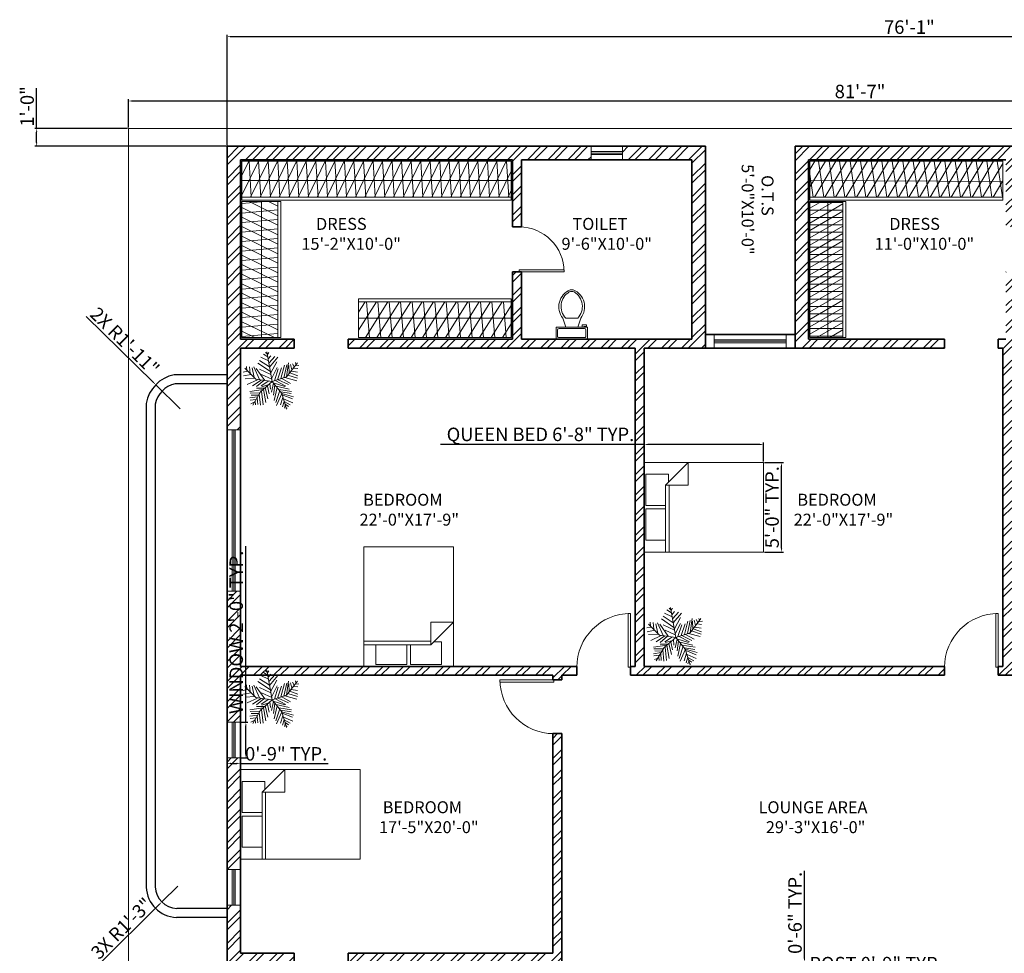
# Model space of a CAD drawing. Units: inches. Extents: x 155 to 1269, y 1260 to 2528.
# Tile 5 of 6: x 155 to 813, y 1903 to 2528. Entities that reach past the tile are written whole.
import ezdxf

# ---------------------------------------------------------------- set-up
doc = ezdxf.new("R2010")
doc.units = ezdxf.units.IN
for name, color, linetype, lineweight in [('A-ANNO-DIMS', 2, 'Continuous', 18), ('A-AREA-IDEN', 7, 'Continuous', 18), ('A-DOOR', 3, 'Continuous', 18), ('A-FLOR-CASE', 9, 'Continuous', 18), ('A-FLOR-CASE-PATT', 252, 'Continuous', 13), ('A-FLOR-EDGE', 7, 'Continuous', 25), ('A-FLOR-FIXT', 9, 'Continuous', 18), ('A-FURN', 8, 'Continuous', 18), ('A-GLAZ', 244, 'Continuous', 18), ('A-WALL', 7, 'Continuous', 35), ('A-WALL-PATT', 252, 'Continuous', 13), ('C-PROP', 8, 'Continuous', 18), ('L-PLNT', 94, 'Continuous', 13)]:
    doc.layers.add(name, color=color, linetype=linetype, lineweight=lineweight)
doc.styles.get("Standard").update_dxf_attribs({"font": 'arial.ttf'})
doc.dimstyles.new('ISO-25', dxfattribs={"dimtxt": 9, "dimasz": 2.5, "dimexe": 1.25, "dimexo": 0.625, "dimtad": 1, "dimlunit": 3, "dimtxsty": 'Standard', "dimcen": 2.5, "dimadec": 0, "dimazin": 0, "dimtfac": 1, "dimtmove": 0, "dimatfit": 3, "dimfxl": 1, "dimarcsym": 0})

# ---------------------------------------------------------------- blocks, each defined once
blk = doc.blocks.new('*U2')
for p, q in [((0, 0), (0, -6)), ((-40, 0), (-40, -6))]:
    blk.add_line(p, q)
blk.add_lwpolyline([(0, 0), (0, 40), (-1.75, 40), (-1.75, 0)], close=True)
blk.add_arc((0, 0), 40, 90, 180)
blk = doc.blocks.new('Bed - Queen')
for p, q in [((0, -80.00003), (0, 0)), ((0, 0), (59.99999, 0)), ((59.99999, 0), (59.99999, -80.00003)), ((7.99999, -1.2), (28.79998, -1.2)), ((7.99999, -14.4), (7.99999, -1.2)), ((28.79998, -1.2), (28.79998, -14.4)), ((31.19999, -1.2), (51.99999, -1.2)), ((31.19999, -14.4), (31.19999, -1.2)), ((51.99999, -1.2), (51.99999, -16.4)), ((0, -14.4), (44.8, -14.4)), ((44.8, -16.8), (0, -16.8)), ((59.99999, -29.6), (44.8, -14.4)), ((44.8, -14.4), (44.8, -29.6)), ((51.99999, -16.4), (46.79936, -16.4)), ((44.8, -29.6), (59.99999, -29.6)), ((59.99999, -80.00003), (0, -80.00003))]:
    blk.add_line(p, q)
blk = doc.blocks.new('*U8')
for p, q in [((9.5, -6), (9.5, -2)), ((-10, -8.5), (-8, -8.5)), ((-10, -9.5), (-10, -8.5)), ((-7, -9.5), (-10, -9.5)), ((-8, -8.5), (-8, -8)), ((-7, -8), (-7, -9.5)), ((-4, -8), (-6, -14)), ((4, -8), (6, -14)), ((4, -14), (-4, -14))]:
    blk.add_line(p, q)
blk.add_lwpolyline([(10.5, -8), (10.5, 0), (-10.5, 0), (-10.5, -8)], close=True)
for points in [[(-9.5, -2), (-9.5, -6)], [(8.5, -1), (-8.5, -1)], [(-8.5, -7), (8.5, -7)]]:
    blk.add_lwpolyline(points)
for centre, radius, start, end in [((-8.62, -1.88), 0.884, 81.8699, 188.1301), ((-8.62, -6.12), 0.884, 171.8699, 278.1301), ((8.62, -1.88), 0.884, 351.8699, 98.1301), ((8.62, -6.12), 0.884, 261.8699, 8.1301), ((3.52, -21.58), 12.17, 141.46911, 247.97143), ((4.2, -21.82), 11.33, 136.36773, 238.94682), ((-3.52, -21.58), 12.17, 292.02843, 38.53071), ((-4.2, -21.82), 11.33, 301.05301, 43.63209), ((0, -27.88), 4, 245.73182, 294.26817), ((0, -29), 4, 254.86053, 285.13947)]:
    blk.add_arc(centre, radius, start, end)
blk = doc.blocks.new('*U11')
for p, q in [((0, 0), (-10.5, 57)), ((-5.114, 28.097), (-24.676, 40.636)), ((-7.288, 39.707), (-21.778, 46.673)), ((-8.737, 47.138), (-17.069, 52.711)), ((-10.186, 53.64), (-13.084, 55.962)), ((-9.099, 51.782), (-6.563, 55.962)), ((-7.65, 43.423), (-2.578, 49.46)), ((-5.839, 35.992), (4.667, 48.067)), ((-5.114, 27.632), (10.463, 46.673)), ((-2.941, 16.486), (8.652, 37.85)), ((-47.498, 19.737), (-55.83, 18.344)), ((-31.5, 4.5), (-52.5, 25.5)), ((-48.585, 21.131), (-49.309, 29.026)), ((-43.513, 28.561), (-42.427, 15.558)), ((-38.442, 26.239), (-34.819, 7.663)), ((-35.544, 28.097), (-24.314, 3.947)), ((-14.533, 2.09), (-30.834, 25.31)), ((-3.665, 19.273), (-27.574, 35.527)), ((-24.314, 23.917), (-2.941, 13.7)), ((-1.129, 6.734), (9.014, 26.704)), ((3.942, 1.625), (11.187, 24.381)), ((10.101, 3.483), (17.708, 26.239)), ((16.259, 5.805), (23.142, 31.348)), ((22.055, 7.198), (27.489, 32.277)), ((27, 9), (48, 36)), ((27.127, 9.056), (31.112, 35.992)), ((31.836, 30.883), (32.561, 16.486)), ((35.096, 32.741), (37.27, 22.524)), ((36.183, 19.737), (48.137, 17.88)), ((38.719, 34.134), (41.979, 28.561)), ((40.53, 25.775), (48.862, 24.846)), ((43.791, 29.954), (51.036, 30.883)), ((44.153, 36.456), (45.239, 32.741)), ((-40.615, 13.7), (-55.105, 10.913)), ((-33.37, 6.269), (-52.207, 5.34)), ((-28.299, 3.483), (-47.86, -5.805)), ((-21.416, 3.018), (-38.079, -8.128)), ((0, 0), (-31.5, 4.5)), ((-15.982, 2.09), (-30.11, -9.521)), ((0, 0), (-22.5, -19.5)), ((-6.563, 1.161), (-21.416, -8.128)), ((-20.691, 13.7), (-1.129, 4.876)), ((0, 0), (27, 9)), ((0, 0), (18, -22.5)), ((6.478, 1.625), (26.04, -8.592)), ((11.187, 3.483), (30.749, -5.805)), ((18.07, 5.805), (35.096, -3.483)), ((24.229, 7.663), (46.688, 1.625)), ((29.662, 12.307), (48.137, 6.269)), ((33.285, 16.486), (48.862, 10.913)), ((-17.431, -15.094), (-42.789, -18.809)), ((-15.257, -12.772), (-30.11, -12.772)), ((-20.691, -18.345), (-17.793, -44.352)), ((-6.563, -5.805), (-19.967, -9.985)), ((-17.069, -15.094), (-12.721, -40.172)), ((-13.446, -11.378), (-8.737, -32.741)), ((-9.461, -8.592), (-6.201, -23.453)), ((-4.752, -3.483), (-3.665, -14.629)), ((2.493, -3.019), (-1.491, -20.202)), ((1.769, -2.555), (24.229, -9.521)), ((5.029, -6.27), (2.131, -25.775)), ((9.014, -11.378), (3.58, -35.992)), ((14.085, -16.951), (6.478, -40.172)), ((7.565, -9.056), (32.198, -14.629)), ((12.274, -15.094), (36.907, -18.809)), ((-28.299, -29.026), (-42.789, -31.348)), ((-24.314, -21.596), (-42.427, -22.06)), ((-30.834, -34.135), (-42.427, -35.528)), ((-26.849, -26.24), (-40.253, -25.775)), ((-22.5, -19.5), (-37.5, -45)), ((-32.646, -36.921), (-31.921, -44.352)), ((-29.023, -30.884), (-27.936, -43.887)), ((-25.038, -23.918), (-22.865, -45.281)), ((18.07, -22.524), (8.289, -45.745)), ((20.244, -30.419), (15.897, -44.816)), ((16.259, -19.738), (36.183, -22.989)), ((18, -22.5), (27, -52.5)), ((18.433, -22.524), (40.53, -29.026)), ((19.157, -25.311), (38.719, -33.206)), ((21.331, -32.741), (39.081, -40.636)), ((-34.457, -39.708), (-40.978, -42.494)), ((22.78, -37.85), (19.519, -48.532)), ((22.78, -38.314), (34.372, -44.816)), ((24.591, -45.745), (23.142, -50.854)), ((24.591, -43.423), (30.749, -47.603)), ((26.764, -49.925), (28.213, -50.854))]:
    blk.add_line(p, q)
blk = doc.blocks.new('*D12')
at = {"layer": 'A-ANNO-DIMS', "color": 0, "lineweight": -2, "transparency": 16777216}
for p, q in [((227.4, 2455.81), (227.4, 2474.72)), ((1203.9, 2473.47), (229.9, 2473.47)), ((1206.4, 2455.81), (1206.4, 2474.72))]:
    blk.add_line(p, q, dxfattribs=at)
at = {"layer": 'A-ANNO-DIMS', "color": 0, "transparency": 16777216}
for points in [[(229.9, 2473.89), (229.9, 2473.06), (227.4, 2473.47)], [(1203.9, 2473.89), (1203.9, 2473.06), (1206.4, 2473.47)]]:
    blk.add_solid(points, dxfattribs=at)
at = {"layer": 'Defpoints', "color": 0, "transparency": 16777216}
for p in [(227.4, 2473.47), (227.4, 2455.18), (1206.4, 2455.18)]:
    blk.add_point(p, dxfattribs=at)
at = {"layer": 'A-ANNO-DIMS', "color": 0, "transparency": 16777216, "insert": (716.9, 2478.69), "char_height": 9, "attachment_point": 5}
blk.add_mtext('81\'-7"', dxfattribs=at)
blk = doc.blocks.new('WIN-21IN')
for p, q in [((21, 5.5), (0, 5.5)), ((21, 4.5), (0, 4.5)), ((21, 3.5), (0, 3.5))]:
    blk.add_line(p, q)
blk.add_lwpolyline([(0, 9), (21, 9), (21, 0), (0, 0)], close=True)
blk = doc.blocks.new('WIN-108IN')
for p, q in [((3.5, 108), (3.5, 0)), ((4.5, 108), (4.5, 0)), ((5.5, 108), (5.5, 0))]:
    blk.add_line(p, q)
blk.add_lwpolyline([(9, 108), (9, 0), (0, 0), (0, 108)], close=True)
blk = doc.blocks.new('WIN-24IN')
for p, q in [((3.5, 24), (3.5, 0)), ((4.5, 24), (4.5, 0)), ((5.5, 24), (5.5, 0))]:
    blk.add_line(p, q)
blk.add_lwpolyline([(0, 24), (9, 24), (9, 0), (0, 0)], close=True)
blk = doc.blocks.new('WIN-48IN')
for p, q in [((0, 5.5), (48, 5.5)), ((0, 4.5), (48, 4.5)), ((0, 3.5), (48, 3.5))]:
    blk.add_line(p, q)
blk.add_lwpolyline([(0, 9), (48, 9), (48, 0), (0, 0)], close=True)
blk = doc.blocks.new('*D22')
at = {"layer": 'A-ANNO-DIMS', "color": 0, "lineweight": -2, "transparency": 16777216}
for p, q in [((572.4, 2243.68), (436.26, 2243.68)), ((572.4, 2232.31), (572.4, 2244.93)), ((649.9, 2243.68), (574.9, 2243.68)), ((652.4, 2232.31), (652.4, 2244.93))]:
    blk.add_line(p, q, dxfattribs=at)
at = {"layer": 'A-ANNO-DIMS', "color": 0, "transparency": 16777216}
for points in [[(574.9, 2244.1), (574.9, 2243.26), (572.4, 2243.68)], [(649.9, 2244.1), (649.9, 2243.26), (652.4, 2243.68)]]:
    blk.add_solid(points, dxfattribs=at)
at = {"layer": 'Defpoints', "color": 0, "transparency": 16777216}
for p in [(572.4, 2243.68), (572.4, 2231.68), (652.4, 2231.68)]:
    blk.add_point(p, dxfattribs=at)
at = {"layer": 'A-ANNO-DIMS', "color": 0, "transparency": 16777216, "insert": (503.08, 2249.24), "char_height": 9, "attachment_point": 5}
blk.add_mtext('QUEEN BED 6\'-8" TYP.', dxfattribs=at)
blk = doc.blocks.new('*D23')
at = {"layer": 'A-ANNO-DIMS', "color": 0, "lineweight": -2, "transparency": 16777216}
for p, q in [((653.02, 2231.68), (665.65, 2231.68)), ((664.4, 2174.18), (664.4, 2229.18)), ((653.02, 2171.68), (665.65, 2171.68))]:
    blk.add_line(p, q, dxfattribs=at)
at = {"layer": 'A-ANNO-DIMS', "color": 0, "transparency": 16777216}
for points in [[(663.98, 2229.18), (664.81, 2229.18), (664.4, 2231.68)], [(663.98, 2174.18), (664.81, 2174.18), (664.4, 2171.68)]]:
    blk.add_solid(points, dxfattribs=at)
at = {"layer": 'Defpoints', "color": 0, "transparency": 16777216}
for p in [(652.4, 2231.68), (664.4, 2231.68), (652.4, 2171.68)]:
    blk.add_point(p, dxfattribs=at)
at = {"layer": 'A-ANNO-DIMS', "color": 0, "transparency": 16777216, "insert": (659.18, 2201.68), "char_height": 9, "attachment_point": 5, "rotation": 90}
blk.add_mtext('5\'-0" TYP.', dxfattribs=at)
blk = doc.blocks.new('*D26')
at = {"layer": 'A-ANNO-DIMS', "color": 0, "lineweight": -2, "transparency": 16777216}
for p, q in [((669.4, 1890.56), (669.4, 1888.58)), ((678.4, 1890.56), (678.4, 1888.58)), ((671.9, 1889.83), (675.9, 1889.83)), ((678.4, 1889.83), (774.28, 1889.83))]:
    blk.add_line(p, q, dxfattribs=at)
at = {"layer": 'A-ANNO-DIMS', "color": 0, "transparency": 16777216}
for points in [[(671.9, 1890.25), (671.9, 1889.41), (669.4, 1889.83)], [(675.9, 1890.25), (675.9, 1889.41), (678.4, 1889.83)]]:
    blk.add_solid(points, dxfattribs=at)
at = {"layer": 'Defpoints', "color": 0, "transparency": 16777216}
for p in [(669.4, 1891.18), (678.4, 1891.18), (678.4, 1889.83)]:
    blk.add_point(p, dxfattribs=at)
at = {"layer": 'A-ANNO-DIMS', "color": 0, "transparency": 16777216, "insert": (727.59, 1895.11), "char_height": 9, "attachment_point": 5}
blk.add_mtext('POST 0\'-9" TYP.', dxfattribs=at)
blk = doc.blocks.new('*D27')
at = {"layer": 'A-ANNO-DIMS', "color": 0, "lineweight": -2, "transparency": 16777216}
for p, q in [((679.75, 1899.68), (679.75, 1958.29)), ((679.02, 1897.18), (681, 1897.18)), ((679.75, 1891.18), (679.75, 1897.18)), ((679.02, 1891.18), (681, 1891.18)), ((679.75, 1888.68), (679.75, 1886.18))]:
    blk.add_line(p, q, dxfattribs=at)
at = {"layer": 'A-ANNO-DIMS', "color": 0, "transparency": 16777216}
for points in [[(679.33, 1899.68), (680.16, 1899.68), (679.75, 1897.18)], [(679.33, 1888.68), (680.16, 1888.68), (679.75, 1891.18)]]:
    blk.add_solid(points, dxfattribs=at)
at = {"layer": 'Defpoints', "color": 0, "transparency": 16777216}
for p in [(678.4, 1897.18), (679.75, 1897.18), (678.4, 1891.18)]:
    blk.add_point(p, dxfattribs=at)
at = {"layer": 'A-ANNO-DIMS', "color": 0, "transparency": 16777216, "insert": (674.53, 1930.24), "char_height": 9, "attachment_point": 5, "rotation": 90}
blk.add_mtext('0\'-6" TYP.', dxfattribs=at)
blk = doc.blocks.new('*D32')
at = {"layer": 'A-ANNO-DIMS', "color": 0, "lineweight": -2, "transparency": 16777216}
for p, q in [((306, 2057.89), (306, 2175.53)), ((303.02, 2057.89), (307.25, 2057.89)), ((306, 2036.39), (306, 2055.39)), ((303.02, 2033.89), (307.25, 2033.89))]:
    blk.add_line(p, q, dxfattribs=at)
at = {"layer": 'A-ANNO-DIMS', "color": 0, "transparency": 16777216}
for points in [[(305.58, 2055.39), (306.41, 2055.39), (306, 2057.89)], [(305.58, 2036.39), (306.41, 2036.39), (306, 2033.89)]]:
    blk.add_solid(points, dxfattribs=at)
at = {"layer": 'Defpoints', "color": 0, "transparency": 16777216}
for p in [(302.4, 2057.89), (306, 2057.89), (302.4, 2033.89)]:
    blk.add_point(p, dxfattribs=at)
at = {"layer": 'A-ANNO-DIMS', "color": 0, "transparency": 16777216, "insert": (300.72, 2117.96), "char_height": 9, "attachment_point": 5, "rotation": 90}
blk.add_mtext('WINDOW 2\'-0" TYP.', dxfattribs=at)
blk = doc.blocks.new('*D33')
at = {"layer": 'A-ANNO-DIMS', "color": 0, "lineweight": -2, "transparency": 16777216}
for p, q in [((293.4, 2033.27), (293.4, 2029.04)), ((295.9, 2030.29), (299.9, 2030.29)), ((302.4, 2033.27), (302.4, 2029.04)), ((302.4, 2030.29), (361.01, 2030.29))]:
    blk.add_line(p, q, dxfattribs=at)
at = {"layer": 'A-ANNO-DIMS', "color": 0, "transparency": 16777216}
for points in [[(295.9, 2030.71), (295.9, 2029.87), (293.4, 2030.29)], [(299.9, 2030.71), (299.9, 2029.87), (302.4, 2030.29)]]:
    blk.add_solid(points, dxfattribs=at)
at = {"layer": 'Defpoints', "color": 0, "transparency": 16777216}
for p in [(293.4, 2033.89), (302.4, 2033.89), (302.4, 2030.29)]:
    blk.add_point(p, dxfattribs=at)
at = {"layer": 'A-ANNO-DIMS', "color": 0, "transparency": 16777216, "insert": (332.95, 2035.51), "char_height": 9, "attachment_point": 5}
blk.add_mtext('0\'-9" TYP.', dxfattribs=at)
blk = doc.blocks.new('*D42')
at = {"layer": 'A-ANNO-DIMS', "color": 0, "lineweight": -2, "transparency": 16777216}
for p, q in [((293.4, 2443.81), (293.4, 2517.78)), ((295.9, 2516.53), (1203.9, 2516.53)), ((1206.4, 2443.81), (1206.4, 2517.78))]:
    blk.add_line(p, q, dxfattribs=at)
at = {"layer": 'A-ANNO-DIMS', "color": 0, "transparency": 16777216}
for points in [[(295.9, 2516.95), (295.9, 2516.11), (293.4, 2516.53)], [(1203.9, 2516.95), (1203.9, 2516.11), (1206.4, 2516.53)]]:
    blk.add_solid(points, dxfattribs=at)
at = {"layer": 'Defpoints', "color": 0, "transparency": 16777216}
for p in [(1206.4, 2516.53), (293.4, 2443.18), (1206.4, 2443.18)]:
    blk.add_point(p, dxfattribs=at)
at = {"layer": 'A-ANNO-DIMS', "color": 0, "transparency": 16777216, "insert": (749.9, 2521.75), "char_height": 9, "attachment_point": 5}
blk.add_mtext('76\'-1"', dxfattribs=at)
blk = doc.blocks.new('*D43')
at = {"layer": 'A-ANNO-DIMS', "color": 0, "lineweight": -2, "transparency": 16777216}
for p, q in [((166.05, 2455.18), (166.05, 2482.01)), ((226.77, 2455.18), (164.8, 2455.18)), ((166.05, 2445.68), (166.05, 2452.68)), ((292.77, 2443.18), (164.8, 2443.18))]:
    blk.add_line(p, q, dxfattribs=at)
at = {"layer": 'A-ANNO-DIMS', "color": 0, "transparency": 16777216}
for points in [[(165.63, 2452.68), (166.46, 2452.68), (166.05, 2455.18)], [(165.63, 2445.68), (166.46, 2445.68), (166.05, 2443.18)]]:
    blk.add_solid(points, dxfattribs=at)
at = {"layer": 'Defpoints', "color": 0, "transparency": 16777216}
for p in [(166.05, 2455.18), (227.4, 2455.18), (293.4, 2443.18)]:
    blk.add_point(p, dxfattribs=at)
at = {"layer": 'A-ANNO-DIMS', "color": 0, "transparency": 16777216, "insert": (160.83, 2469.84), "char_height": 9, "attachment_point": 5, "rotation": 90}
blk.add_mtext('1\'-0"', dxfattribs=at)
blk = doc.blocks.new('*D50')
at = {"layer": 'A-ANNO-DIMS', "color": 0, "lineweight": -2, "transparency": 16777216}
for p, q in [((199.11, 2329.37), (243.91, 2285.4)), ((262.1, 2267.55), (245.69, 2283.65))]:
    blk.add_line(p, q, dxfattribs=at)
at = {"layer": 'A-ANNO-DIMS', "color": 0, "transparency": 16777216}
blk.add_solid([(244.2, 2285.7), (243.62, 2285.1), (245.69, 2283.65)], dxfattribs=at)
at = {"layer": 'Defpoints', "color": 0, "transparency": 16777216}
for p in [(245.69, 2283.65), (262.1, 2267.55)]:
    blk.add_point(p, dxfattribs=at)
at = {"layer": 'A-ANNO-DIMS', "color": 0, "transparency": 16777216, "insert": (224.22, 2311.93), "char_height": 9, "attachment_point": 5, "rotation": 315.54002}
blk.add_mtext('2X R1\'-11"', dxfattribs=at)
blk = doc.blocks.new('*D56')
at = {"layer": 'A-ANNO-DIMS', "color": 0, "lineweight": -2, "transparency": 16777216}
for p, q in [((260.38, 1948.16), (249.76, 1937.58)), ((208.58, 1896.56), (247.98, 1935.81))]:
    blk.add_line(p, q, dxfattribs=at)
at = {"layer": 'A-ANNO-DIMS', "color": 0, "transparency": 16777216}
blk.add_solid([(247.69, 1936.11), (248.28, 1935.52), (249.76, 1937.58)], dxfattribs=at)
at = {"layer": 'Defpoints', "color": 0, "transparency": 16777216}
for p in [(260.38, 1948.16), (249.76, 1937.58)]:
    blk.add_point(p, dxfattribs=at)
at = {"layer": 'A-ANNO-DIMS', "color": 0, "transparency": 16777216, "insert": (223.71, 1919), "char_height": 9, "attachment_point": 5, "rotation": 44.89223}
blk.add_mtext('3X R1\'-3"', dxfattribs=at)

msp = doc.modelspace()

# ---------------------------------------------------------------- hatches: boundary and pattern name
at = {"layer": 'A-FLOR-CASE-PATT'}
h = msp.add_hatch(dxfattribs=at)
h.set_pattern_fill('ANSI31', color=256, scale=1.80661, angle=19.0965, style=0)
h.paths.add_polyline_path([(303.397, 2409.181), (483.397, 2409.181), (483.397, 2433.181), (303.397, 2433.181)])
h = msp.add_hatch(dxfattribs=at)
h.set_pattern_fill('ANSI31', color=256, scale=2.00453, angle=48.55, style=0)
h.paths.add_polyline_path([(303.397, 2409.181), (483.397, 2409.181), (483.397, 2433.181), (303.397, 2433.181)])
h = msp.add_hatch(dxfattribs=at)
h.set_pattern_fill('ANSI31', color=256, scale=1.89921, angle=14.0303, style=0)
h.paths.add_polyline_path([(683.397, 2409.181), (812.397, 2409.181), (812.397, 2433.181), (683.397, 2433.181)])
h = msp.add_hatch(dxfattribs=at)
h.set_pattern_fill('ANSI31', color=256, scale=2.1922, angle=53.2238, style=0)
h.paths.add_polyline_path([(683.397, 2409.181), (812.397, 2409.181), (812.397, 2433.181), (683.397, 2433.181)])
h = msp.add_hatch(dxfattribs=at)
h.set_pattern_fill('ANSI31', color=256, scale=1.799134, angle=108.8969, style=0)
h.paths.add_polyline_path([(303.397, 2315.181), (327.397, 2315.181), (327.397, 2406.181), (303.397, 2406.181)])
h = msp.add_hatch(dxfattribs=at)
h.set_pattern_fill('ANSI31', color=256, scale=1.99625, angle=-40.1304, style=0)
h.paths.add_polyline_path([(303.397, 2315.181), (327.397, 2315.181), (327.397, 2406.181), (303.397, 2406.181)])
h = msp.add_hatch(dxfattribs=at)
h.set_pattern_fill('ANSI31', color=256, scale=1.349876, angle=-14.7838, style=0)
h.paths.add_polyline_path([(683.397, 2315.181), (705.397, 2315.181), (705.397, 2406.181), (683.397, 2406.181)])
h = msp.add_hatch(dxfattribs=at)
h.set_pattern_fill('ANSI31', color=256, scale=1.562117, angle=-45, style=0)
h.paths.add_polyline_path([(683.397, 2315.181), (705.397, 2315.181), (705.397, 2406.181), (683.397, 2406.181)])
h = msp.add_hatch(dxfattribs=at)
h.set_pattern_fill('ANSI31', color=256, scale=2.03916, angle=12.988, style=0)
h.paths.add_polyline_path([(381.458, 2315.181), (483.397, 2315.181), (483.397, 2339.181), (381.458, 2339.181)])
h = msp.add_hatch(dxfattribs=at)
h.set_pattern_fill('ANSI31', color=256, scale=2.39665, angle=49.7328, style=0)
h.paths.add_polyline_path([(381.458, 2315.181), (483.397, 2315.181), (483.397, 2339.181), (381.458, 2339.181)])
at = {"layer": 'A-WALL-PATT'}
h = msp.add_hatch(dxfattribs=at)
h.set_pattern_fill('ANSI32', color=256)
h.paths.add_polyline_path([(614.897, 1534.181), (593.397, 1534.181), (593.397, 1555.181), (589.397, 1555.181), (589.397, 1534.181), (517.397, 1534.181), (517.397, 1555.181), (511.397, 1555.181), (511.397, 1495.181), (488.631, 1495.181), (488.631, 1486.181), (517.397, 1486.181), (517.397, 1525.181), (614.897, 1525.181)])
h.paths.add_polyline_path([(440.631, 1495.181), (344.954, 1495.181), (344.954, 1486.181), (440.631, 1486.181)])
h.paths.add_polyline_path([(323.954, 1495.181), (302.397, 1495.181), (302.397, 1625.863), (332.397, 1625.863), (332.397, 1631.863), (302.397, 1631.863), (302.397, 1634.984), (293.397, 1634.984), (293.397, 1486.181), (323.954, 1486.181)])
h.paths.add_polyline_path([(302.397, 1753.181), (386.397, 1753.181), (386.397, 1726.181), (392.397, 1726.181), (392.397, 1753.181), (511.397, 1753.181), (511.397, 1693.181), (392.397, 1693.181), (392.397, 1696.181), (386.397, 1696.181), (386.397, 1693.181), (368.397, 1693.181), (368.397, 1687.181), (511.397, 1687.181), (511.397, 1663.181), (517.397, 1663.181), (517.397, 1891.181), (539.397, 1891.181), (539.397, 1897.181), (517.397, 1897.181), (517.397, 2050.181), (511.397, 2050.181), (511.397, 1903.181), (374.397, 1903.181), (374.397, 1897.181), (410.397, 1897.181), (410.397, 1843.181), (416.397, 1843.181), (416.397, 1897.181), (511.397, 1897.181), (511.397, 1759.181), (416.397, 1759.181), (416.397, 1813.181), (410.397, 1813.181), (410.397, 1759.181), (302.397, 1759.181), (302.397, 1897.181), (338.397, 1897.181), (338.397, 1903.181), (302.397, 1903.181), (302.397, 1935.29), (293.397, 1935.29), (293.397, 1682.984), (302.397, 1682.984), (302.397, 1687.181), (338.397, 1687.181), (338.397, 1693.181), (302.397, 1693.181)])
h.paths.add_polyline_path([(645.397, 1897.181), (623.397, 1897.181), (623.397, 1891.181), (645.397, 1891.181)])
h.paths.add_polyline_path([(678.397, 1897.181), (669.397, 1897.181), (669.397, 1891.181), (678.397, 1891.181)])
h.paths.add_polyline_path([(696.397, 1897.181), (687.397, 1897.181), (687.397, 1891.181), (696.397, 1891.181)])
h.paths.add_polyline_path([(714.397, 1897.181), (705.397, 1897.181), (705.397, 1891.181), (714.397, 1891.181)])
h.paths.add_polyline_path([(732.397, 1897.181), (723.397, 1897.181), (723.397, 1891.181), (732.397, 1891.181)])
h.paths.add_polyline_path([(302.397, 2033.891), (293.397, 2033.891), (293.397, 1959.29), (302.397, 1959.29)], flags=17)
h.paths.add_polyline_path([(302.397, 2089.181), (511.397, 2089.181), (511.397, 2086.181), (517.397, 2086.181), (517.397, 2089.181), (527.397, 2089.181), (527.397, 2095.181), (302.397, 2095.181), (302.397, 2145.471), (293.397, 2145.471), (293.397, 2057.891), (302.397, 2057.891)])
h.paths.add_polyline_path([(773.397, 2095.181), (572.397, 2095.181), (572.397, 2308.181), (613.397, 2308.181), (613.397, 2443.181), (557.897, 2443.181), (557.897, 2434.181), (604.397, 2434.181), (604.397, 2314.181), (490.397, 2314.181), (490.397, 2359.181), (484.397, 2359.181), (484.397, 2314.181), (374.397, 2314.181), (374.397, 2308.181), (566.397, 2308.181), (566.397, 2095.181), (563.397, 2095.181), (563.397, 2089.181), (773.397, 2089.181)])
h.paths.add_polyline_path([(1070.397, 2147.681), (1061.397, 2147.681), (1061.397, 2095.181), (857.397, 2095.181), (857.397, 2089.181), (868.397, 2089.181), (868.397, 2086.181), (874.397, 2086.181), (874.397, 2089.181), (1061.397, 2089.181), (1061.397, 2050.181), (1070.397, 2050.181)])
h.paths.add_polyline_path([(821.397, 2095.181), (818.397, 2095.181), (818.397, 2308.181), (1022.397, 2308.181), (1022.397, 2314.181), (940.397, 2314.181), (940.397, 2434.181), (1077.397, 2434.181), (1077.397, 2389.181), (1083.397, 2389.181), (1083.397, 2434.181), (1129.897, 2434.181), (1129.897, 2443.181), (887.897, 2443.181), (887.897, 2434.181), (934.397, 2434.181), (934.397, 2314.181), (820.397, 2314.181), (820.397, 2359.181), (814.397, 2359.181), (814.397, 2314.181), (809.397, 2314.181), (809.397, 2308.181), (812.397, 2308.181), (812.397, 2095.181), (809.397, 2095.181), (809.397, 2089.181), (821.397, 2089.181)])
h.paths.add_polyline_path([(874.397, 2050.181), (868.397, 2050.181), (868.397, 1741.181), (877.397, 1741.181), (877.397, 1747.181), (892.397, 1747.181), (892.397, 1753.181), (874.397, 1753.181), (874.397, 1819.181), (940.397, 1819.181), (940.397, 1753.181), (922.397, 1753.181), (922.397, 1747.181), (946.397, 1747.181), (946.397, 1819.181), (1151.397, 1819.181), (1151.397, 1683.181), (931.397, 1683.181), (931.397, 1677.181), (1064.397, 1677.181), (1064.397, 1495.181), (877.397, 1495.181), (877.397, 1638.181), (868.397, 1638.181), (868.397, 1534.181), (796.397, 1534.181), (796.397, 1555.181), (792.397, 1555.181), (792.397, 1534.181), (770.897, 1534.181), (770.897, 1525.181), (868.397, 1525.181), (868.397, 1486.181), (1073.397, 1486.181), (1073.397, 1677.181), (1160.397, 1677.181), (1160.397, 1825.181), (1070.397, 1825.181), (1070.397, 1942.181), (1061.397, 1942.181), (1061.397, 1903.181), (913.397, 1903.181), (913.397, 1897.181), (1061.397, 1897.181), (1061.397, 1825.181), (957.406, 1825.181), (957.406, 1861.181), (951.406, 1861.181), (951.406, 1825.181), (874.397, 1825.181), (874.397, 1897.181), (877.397, 1897.181), (877.397, 1903.181), (874.397, 1903.181)])
h.paths.add_polyline_path([(1070.397, 2305.181), (1206.397, 2305.181), (1206.397, 2443.181), (1150.897, 2443.181), (1150.897, 2434.181), (1197.397, 2434.181), (1197.397, 2314.181), (1083.397, 2314.181), (1083.397, 2359.181), (1077.397, 2359.181), (1077.397, 2314.181), (1058.397, 2314.181), (1058.397, 2308.181), (1061.397, 2308.181), (1061.397, 2255.681), (1070.397, 2255.681)])
h.paths.add_polyline_path([(866.897, 2443.181), (673.397, 2443.181), (673.397, 2308.181), (773.397, 2308.181), (773.397, 2314.181), (682.397, 2314.181), (682.397, 2434.181), (814.397, 2434.181), (814.397, 2389.181), (818.897, 2389.181), (820.397, 2389.181), (820.397, 2434.181), (866.897, 2434.181)])
h.paths.add_polyline_path([(536.897, 2443.181), (293.397, 2443.181), (293.397, 2253.471), (302.397, 2253.471), (302.397, 2308.181), (338.397, 2308.181), (338.397, 2314.181), (302.397, 2314.181), (302.397, 2434.181), (484.397, 2434.181), (484.397, 2389.181), (490.397, 2389.181), (490.397, 2434.181), (536.897, 2434.181)])

# ---------------------------------------------------------------- linework, layer by layer
at = {"layer": 'A-FLOR-CASE'}
for p, q in [((303.397, 2433.181), (483.397, 2433.181)), ((303.397, 2433.181), (303.397, 2407.181)), ((483.397, 2433.181), (483.397, 2407.181)), ((683.397, 2433.181), (812.397, 2433.181)), ((683.397, 2433.181), (683.397, 2407.181)), ((812.397, 2433.181), (812.397, 2407.181)), ((303.397, 2420.181), (483.397, 2420.181)), ((683.397, 2420.181), (812.397, 2419.681)), ((303.397, 2409.181), (483.397, 2409.181)), ((303.397, 2407.181), (483.397, 2407.181)), ((303.397, 2406.181), (329.397, 2406.181)), ((303.397, 2406.181), (303.397, 2315.181)), ((316.397, 2406.181), (316.397, 2315.181)), ((327.397, 2406.181), (327.397, 2315.181)), ((329.397, 2406.181), (329.397, 2315.181)), ((683.397, 2409.181), (812.397, 2409.181)), ((683.397, 2407.181), (812.397, 2407.181)), ((683.397, 2406.181), (707.397, 2406.181)), ((683.397, 2406.181), (683.397, 2315.181)), ((695.397, 2406.181), (695.397, 2315.181)), ((705.397, 2406.181), (705.397, 2315.181)), ((707.397, 2406.181), (707.397, 2315.181)), ((381.458, 2341.181), (483.397, 2341.181)), ((381.458, 2315.181), (381.458, 2341.181)), ((381.458, 2339.181), (483.397, 2339.181)), ((483.397, 2341.181), (483.397, 2315.181)), ((381.458, 2328.181), (483.397, 2328.181)), ((303.397, 2315.181), (329.397, 2315.181)), ((381.458, 2315.181), (483.397, 2315.181)), ((683.397, 2315.181), (707.397, 2315.181))]:
    msp.add_line(p, q, dxfattribs=at)
at = {"layer": 'A-FLOR-EDGE'}
for p, q in [((293.397, 2290.181), (258.058, 2290.181)), ((293.397, 2284.181), (258.631, 2284.181)), ((239.397, 2271.165), (239.397, 1947.446)), ((245.397, 2270.654), (245.397, 1947.556)), ((293.397, 1933.181), (259.719, 1933.181)), ((293.397, 1927.181), (259.599, 1927.181))]:
    msp.add_line(p, q, dxfattribs=at)
for centre, radius, start, end in [((262.105, 2267.546), 22.994, 100.135609, 170.943187), ((262.105, 2267.546), 16.994, 101.795322, 169.461113), ((260.376, 1948.157), 20.991, 181.941445, 267.878551), ((260.376, 1948.157), 14.991, 182.2974, 267.489584)]:
    msp.add_arc(centre, radius, start, end, dxfattribs=at)
at = {"layer": 'A-WALL'}
for p, q in [((293.397, 2443.181), (293.397, 1486.181)), ((293.397, 2443.181), (613.397, 2443.181)), ((613.397, 2443.181), (613.397, 2308.181)), ((673.397, 2443.181), (673.397, 2308.181)), ((673.397, 2443.181), (1206.397, 2443.181)), ((302.397, 2434.181), (302.397, 2314.181)), ((302.397, 2434.181), (484.397, 2434.181)), ((484.397, 2434.181), (484.397, 2389.181)), ((490.397, 2434.181), (490.397, 2389.181)), ((490.397, 2434.181), (604.397, 2434.181)), ((604.397, 2434.181), (604.397, 2314.181)), ((682.397, 2434.181), (682.397, 2314.181)), ((682.397, 2434.181), (814.397, 2434.181)), ((484.397, 2389.181), (490.397, 2389.181)), ((484.397, 2359.181), (490.397, 2359.181)), ((484.397, 2359.181), (484.397, 2314.181)), ((490.397, 2359.181), (490.397, 2314.181)), ((302.397, 2314.181), (338.397, 2314.181)), ((338.397, 2314.181), (338.397, 2308.181)), ((374.397, 2314.181), (374.397, 2308.181)), ((374.397, 2314.181), (484.397, 2314.181)), ((490.397, 2314.181), (604.397, 2314.181)), ((613.397, 2317.181), (673.397, 2317.181)), ((682.397, 2314.181), (773.397, 2314.181)), ((773.397, 2308.181), (773.397, 2314.181)), ((809.397, 2308.181), (809.397, 2314.181)), ((809.397, 2314.181), (814.397, 2314.181)), ((302.397, 2308.181), (338.397, 2308.181)), ((302.397, 2308.181), (302.397, 2095.181)), ((374.397, 2308.181), (566.397, 2308.181)), ((566.397, 2308.181), (566.397, 2095.181)), ((572.397, 2308.181), (572.397, 2095.181)), ((572.397, 2308.181), (773.397, 2308.181)), ((809.397, 2308.181), (812.397, 2308.181)), ((812.397, 2308.181), (812.397, 2095.181)), ((302.397, 2095.181), (527.397, 2095.181)), ((527.397, 2095.181), (527.397, 2089.181)), ((563.397, 2095.181), (563.397, 2089.181)), ((563.397, 2095.181), (566.397, 2095.181)), ((572.397, 2095.181), (773.397, 2095.181)), ((773.397, 2095.181), (773.397, 2089.181)), ((809.397, 2095.181), (809.397, 2089.181)), ((809.397, 2095.181), (812.397, 2095.181)), ((302.397, 2089.181), (511.397, 2089.181)), ((302.397, 2089.181), (302.397, 1903.181)), ((511.397, 2089.181), (511.397, 2086.181)), ((517.397, 2089.181), (517.397, 2086.181)), ((517.397, 2089.181), (527.397, 2089.181)), ((563.397, 2089.181), (773.397, 2089.181)), ((809.397, 2089.181), (821.397, 2089.181)), ((517.397, 2086.181), (511.397, 2086.181)), ((517.397, 2050.181), (511.397, 2050.181)), ((511.397, 2050.181), (511.397, 1903.181)), ((517.397, 2050.181), (517.397, 1897.181)), ((302.397, 1903.181), (338.397, 1903.181)), ((338.397, 1897.181), (338.397, 1903.181)), ((374.397, 1897.181), (374.397, 1903.181)), ((374.397, 1903.181), (511.397, 1903.181))]:
    msp.add_line(p, q, dxfattribs=at)
at = {"layer": 'C-PROP'}
for q in [(227.397, 1339.181), (1206.397, 2455.181)]:
    msp.add_line((227.397, 2455.181), q, dxfattribs=at)

# ---------------------------------------------------------------- block references
at = {"layer": 'A-DOOR'}
for p, xscale, yscale, zscale, rotation in [((488.897, 2359.181), 0.7500000000000114, 0.7500000000000114, 0.7500000000000114, 270), ((511.997, 2086.181), 0.9, 0.9, 0.9, 90)]:
    msp.add_blockref('*U2', p, dxfattribs=dict(at, xscale=xscale, yscale=yscale, zscale=zscale, rotation=rotation))
at = {"layer": 'A-DOOR', "xscale": 0.9, "yscale": 0.9, "zscale": 0.9}
for p in [(563.397, 2094.581), (809.397, 2094.581)]:
    msp.add_blockref('*U2', p, dxfattribs=at)
at = {"layer": 'A-FLOR-FIXT', "rotation": 180}
msp.add_blockref('*U8', (523.996, 2314.181), dxfattribs=at)
at = {"layer": 'A-FURN', "rotation": 90}
for p in [(572.397, 2171.681), (302.397, 1966.181)]:
    msp.add_blockref('Bed - Queen', p, dxfattribs=at)
at = {"layer": 'A-FURN', "xscale": -1, "rotation": 180}
msp.add_blockref('Bed - Queen', (384.897, 2095.181), dxfattribs=at)
at = {"layer": 'A-GLAZ'}
for name, p in [('WIN-21IN', (536.897, 2434.181)), ('WIN-48IN', (619.397, 2308.181)), ('WIN-108IN', (293.397, 2145.471)), ('WIN-24IN', (293.397, 2033.891)), ('WIN-24IN', (293.397, 1935.29))]:
    msp.add_blockref(name, p, dxfattribs=at)
at = {"layer": 'L-PLNT', "xscale": 0.3495173552522817, "yscale": 0.3495173552522817, "zscale": 0.3495173552522817}
for p in [(323.697, 2285.73), (593.697, 2114.546), (323.697, 2072.73)]:
    msp.add_blockref('*U11', p, dxfattribs=at)

# ---------------------------------------------------------------- texts
at = {"layer": 'A-AREA-IDEN', "insert": (659.023, 2431.208), "char_height": 8, "attachment_point": 1, "rotation": 270}
msp.add_mtext_dynamic_manual_height_columns('   O.T.S\\P5\'-0"X10\'-0"', width=56.71156, gutter_width=12.5, heights=[0], dxfattribs=at)
at = {"layer": 'A-AREA-IDEN', "char_height": 8, "attachment_point": 1}
for s, width, insert in [('    DRESS\\P15\'-2"X10\'-0"', 61.72868, (343.148, 2395.252)), ('   TOILET\\P9\'-6"X10\'-0"', 56.71156, (517.166, 2395.252)), ('    DRESS\\P11\'-0"X10\'-0"', 61.72868, (726.667, 2395.252)), (' BEDROOM\\P22\'-0"X17\'-9"', 61.72868, (382.04, 2210.676)), (' BEDROOM\\P22\'-0"X17\'-9"', 61.72868, (672.494, 2210.676)), (' BEDROOM\\P17\'-5"X20\'-0"', 61.72868, (395.109, 2004.921)), ('LOUNGE AREA\\P  29\'-3"X16\'-0"', 81.28846, (648.997, 2004.921))]:
    msp.add_mtext_dynamic_manual_height_columns(s, width=width, gutter_width=12.5, heights=[0], dxfattribs=dict(at, insert=insert))

# ---------------------------------------------------------------- dimensions: what is measured, and where the dimension line sits
at = {"layer": 'A-ANNO-DIMS'}
for base, p1, p2, override, picture, middle in [((1206.397, 2516.531), (293.397, 2443.181), (1206.397, 2443.181), {"dimdec": 1, "dimlfac": 1, "dimrnd": 0, "dimzin": 1, "dimdsep": 46, "dimlunit": 4, "dimfrac": 2}, '*D42', (749.897, 2521.751)), ((227.397, 2473.473), (1206.397, 2455.181), (227.397, 2455.181), {"dimclrd": 0, "dimclre": 0, "dimclrt": 0}, '*D12', (716.897, 2478.693))]:
    dim = msp.add_linear_dim(base=base, p1=p1, p2=p2, dimstyle='ISO-25', override=override, dxfattribs=at)
    dim.commit()
    dim.dimension.update_dxf_attribs({"geometry": picture, "text_midpoint": middle})
dim = msp.add_linear_dim(base=(166.047, 2455.181), p1=(293.397, 2443.181), p2=(227.397, 2455.181), angle=90, dimstyle='ISO-25', override={"dimdec": 1, "dimlfac": 1, "dimrnd": 0, "dimzin": 1, "dimdsep": 46, "dimlunit": 4, "dimfrac": 2}, dxfattribs=at)
dim.commit()
dim.dimension.update_dxf_attribs({"geometry": '*D43', "text_midpoint": (160.827, 2469.844)})
for center, mpoint, text, picture, middle in [((262.105, 2267.546), (245.693, 2283.651), '2X <>', '*D50', (224.22, 2311.934)), ((260.376, 1948.157), (249.756, 1937.577), '3X <>', '*D56', (223.712, 1919.003))]:
    dim = msp.add_radius_dim(center=center, mpoint=mpoint, text=text, dimstyle='ISO-25', override={"dimdec": 1, "dimlfac": 1, "dimrnd": 0, "dimzin": 1, "dimdsep": 46, "dimlunit": 4, "dimfrac": 2}, dxfattribs=at)
    dim.commit()
    dim.dimension.update_dxf_attribs({"geometry": picture, "text_midpoint": middle})
for base, p1, p2, angle, text, picture, middle in [((572.397, 2243.681), (652.397, 2231.681), (572.397, 2231.681), 180, 'QUEEN BED <> TYP.', '*D22', (503.077, 2249.236)), ((664.397, 2231.681), (652.397, 2171.681), (652.397, 2231.681), 90, '<> TYP.', '*D23', (659.177, 2201.681)), ((305.997, 2057.891), (302.397, 2033.891), (302.397, 2057.891), 90, 'WINDOW <> TYP.', '*D32', (300.716, 2117.96)), ((679.747, 1897.181), (678.397, 1891.181), (678.397, 1897.181), 90, '<> TYP.', '*D27', (674.527, 1930.236))]:
    dim = msp.add_linear_dim(base=base, p1=p1, p2=p2, angle=angle, text=text, dimstyle='ISO-25', override={"dimdec": 1, "dimlfac": 1, "dimrnd": 0, "dimzin": 1, "dimdsep": 46, "dimlunit": 4, "dimfrac": 2}, dxfattribs=at)
    dim.commit()
    dim.dimension.update_dxf_attribs({"geometry": picture, "text_midpoint": middle})
for base, p1, p2, text, picture, middle in [((302.397, 2030.291), (293.397, 2033.891), (302.397, 2033.891), '<> TYP.', '*D33', (332.952, 2035.511)), ((678.397, 1889.831), (669.397, 1891.181), (678.397, 1891.181), 'POST <> TYP.', '*D26', (727.591, 1895.112))]:
    dim = msp.add_linear_dim(base=base, p1=p1, p2=p2, text=text, dimstyle='ISO-25', override={"dimdec": 1, "dimlfac": 1, "dimrnd": 0, "dimzin": 1, "dimdsep": 46, "dimlunit": 4, "dimfrac": 2}, dxfattribs=at)
    dim.commit()
    dim.dimension.update_dxf_attribs({"geometry": picture, "text_midpoint": middle})

doc.saveas('drawing.dxf')
